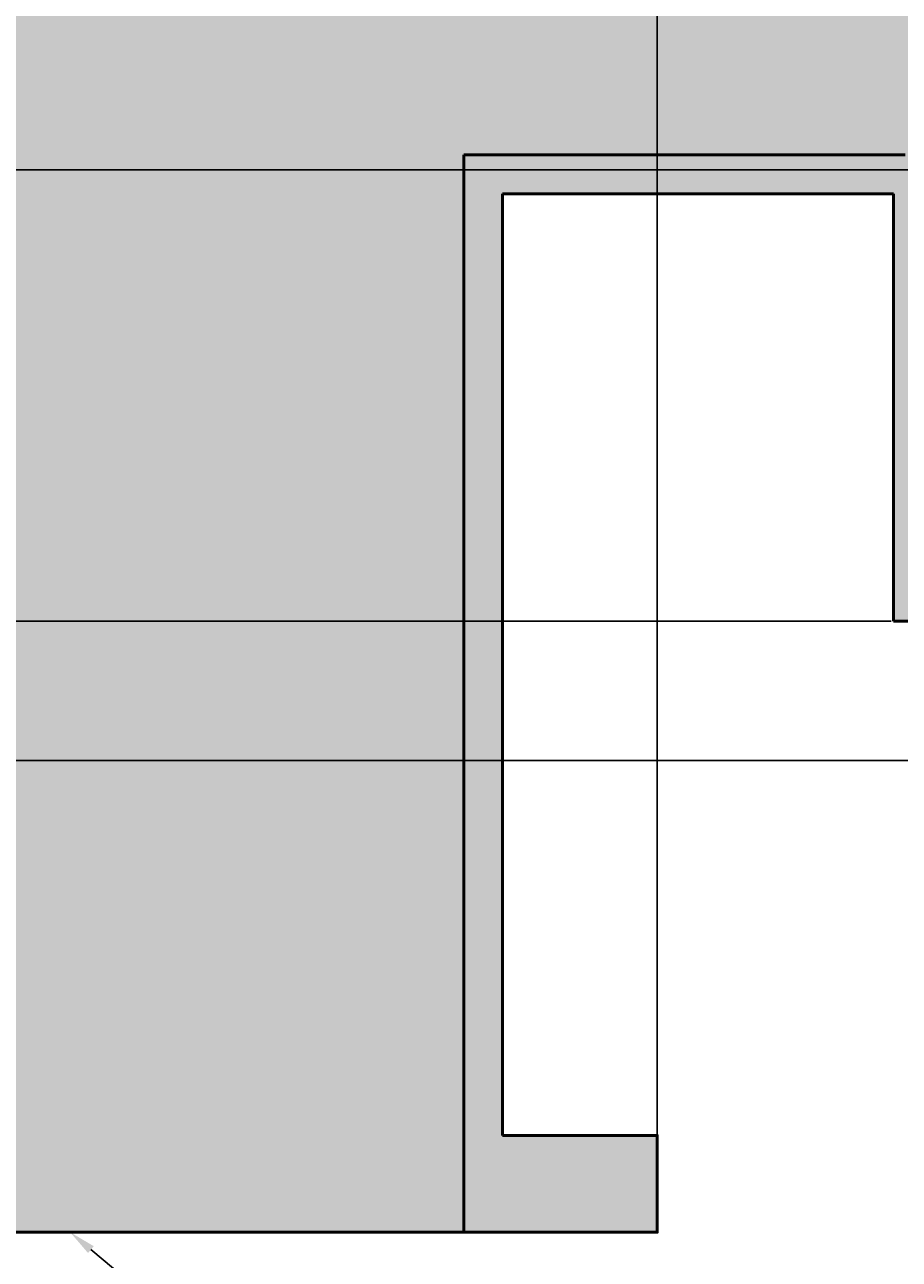
# Model space of a CAD drawing. Units: inches. Extents: x -12 to 334, y -10 to 186.
# Tile 12 of 77: x 42 to 64, y 33 to 65. Entities that reach past the tile are written whole.
import ezdxf
from ezdxf import colors
from ezdxf.entities.mleader import LeaderData, LeaderLine
from ezdxf.math import Vec2, Vec3

# ---------------------------------------------------------------- set-up
doc = ezdxf.new("R2010")
doc.units = ezdxf.units.IN
doc.header["$MEASUREMENT"] = 0
for name, color, linetype, lineweight in [('M-ANNO-TEXT', 3, 'Continuous', 25), ('M-DIMS', 2, 'Continuous', 18), ('M-EQPM', 7, 'Continuous', 50), ('M-EQPM-PATT', 8, 'Continuous', 18)]:
    doc.layers.add(name, color=color, linetype=linetype, lineweight=lineweight)
doc.styles.get("Standard").update_dxf_attribs({"font": 'arial.ttf'})
doc.dimstyles.get("Standard").update_dxf_attribs({"dimtxt": 0.18, "dimasz": 0.18, "dimexe": 0.18, "dimexo": 0.0625, "dimgap": 0.09, "dimtad": 0, "dimtih": 1, "dimtoh": 1, "dimdec": 4, "dimzin": 0, "dimdsep": 46, "dimtxsty": 'Standard', "dimcen": 0.09, "dimadec": 0, "dimazin": 0, "dimtfac": 1, "dimtdec": 4, "dimtofl": 0, "dimtmove": 0, "dimatfit": 3, "dimfxl": 1, "dimtolj": 1, "dimtzin": 0, "dimarcsym": 0})

# ---------------------------------------------------------------- blocks, each defined once
blk = doc.blocks.new('*D1')
at = {"layer": 'Defpoints', "color": 0, "transparency": 16777216}
for p in [(281.426, 91.899), (3.376, 80.692), (281.426, 14.304)]:
    blk.add_point(p, dxfattribs=at)
at = {"layer": 'M-DIMS', "color": 0, "lineweight": -2, "transparency": 16777216}
for p, q in [((281.426, 91.836), (281.426, 14.124)), ((3.376, 80.629), (3.376, 14.124)), ((3.556, 14.304), (141.935, 14.304)), ((281.246, 14.304), (142.867, 14.304))]:
    blk.add_line(p, q, dxfattribs=at)
at = {"layer": 'M-DIMS', "color": 0, "transparency": 16777216}
for points in [[(3.556, 14.334), (3.556, 14.274), (3.376, 14.304)], [(281.246, 14.334), (281.246, 14.274), (281.426, 14.304)]]:
    blk.add_solid(points, dxfattribs=at)
at = {"layer": 'M-DIMS', "color": 0, "transparency": 16777216, "insert": (142.401, 14.304), "char_height": 0.18, "attachment_point": 5}
blk.add_mtext('\\A1;278.05', dxfattribs=at)
blk = doc.blocks.new('*D14')
at = {"layer": 'Defpoints', "color": 0, "transparency": 16777216}
for p in [(63.5, 109.058), (-11.174, 49.45), (64.207, 49.45)]:
    blk.add_point(p, dxfattribs=at)
at = {"layer": 'M-DIMS', "color": 0, "lineweight": -2, "transparency": 16777216}
for p, q in [((63.438, 109.058), (-11.354, 109.058)), ((-11.174, 108.878), (-11.174, 79.436)), ((-11.174, 49.63), (-11.174, 79.072)), ((64.144, 49.45), (-11.354, 49.45))]:
    blk.add_line(p, q, dxfattribs=at)
at = {"layer": 'M-DIMS', "color": 0, "transparency": 16777216}
for points in [[(-11.204, 108.878), (-11.144, 108.878), (-11.174, 109.058)], [(-11.204, 49.63), (-11.144, 49.63), (-11.174, 49.45)]]:
    blk.add_solid(points, dxfattribs=at)
at = {"layer": 'M-DIMS', "color": 0, "transparency": 16777216, "insert": (-11.174, 79.254), "char_height": 0.18, "attachment_point": 5}
blk.add_mtext('\\A1;59.61', dxfattribs=at)
blk = doc.blocks.new('*D26')
at = {"layer": 'Defpoints', "color": 0, "transparency": 16777216}
for p in [(87.888, 169.385), (87.888, 56.321), (58.1, 33.675)]:
    blk.add_point(p, dxfattribs=at)
at = {"layer": 'M-DIMS', "color": 0, "lineweight": -2, "transparency": 16777216}
for p, q in [((58.1, 33.738), (58.1, 169.565)), ((58.28, 169.385), (72.599, 169.385)), ((87.708, 169.385), (73.389, 169.385)), ((87.888, 56.383), (87.888, 169.565))]:
    blk.add_line(p, q, dxfattribs=at)
at = {"layer": 'M-DIMS', "color": 0, "transparency": 16777216}
for points in [[(58.28, 169.415), (58.28, 169.355), (58.1, 169.385)], [(87.708, 169.415), (87.708, 169.355), (87.888, 169.385)]]:
    blk.add_solid(points, dxfattribs=at)
at = {"layer": 'M-DIMS', "color": 0, "transparency": 16777216, "insert": (72.994, 169.385), "char_height": 0.18, "attachment_point": 5}
blk.add_mtext('\\A1;29.79', dxfattribs=at)
blk = doc.blocks.new('*D29')
at = {"layer": 'Defpoints', "color": 0, "transparency": 16777216}
for p in [(-11.174, 45.854), (221.576, 45.854), (216.576, 30.854)]:
    blk.add_point(p, dxfattribs=at)
at = {"layer": 'M-DIMS', "color": 0, "lineweight": -2, "transparency": 16777216}
for p, q in [((221.514, 45.854), (-11.354, 45.854)), ((-11.174, 45.674), (-11.174, 38.536)), ((-11.174, 31.034), (-11.174, 38.172)), ((216.514, 30.854), (-11.354, 30.854))]:
    blk.add_line(p, q, dxfattribs=at)
at = {"layer": 'M-DIMS', "color": 0, "transparency": 16777216}
for points in [[(-11.204, 45.674), (-11.144, 45.674), (-11.174, 45.854)], [(-11.204, 31.034), (-11.144, 31.034), (-11.174, 30.854)]]:
    blk.add_solid(points, dxfattribs=at)
at = {"layer": 'M-DIMS', "color": 0, "transparency": 16777216, "insert": (-11.174, 38.354), "char_height": 0.18, "attachment_point": 5}
blk.add_mtext('\\A1;15', dxfattribs=at)
blk = doc.blocks.new('*D35')
at = {"layer": 'Defpoints', "color": 0, "transparency": 16777216}
for p in [(216.428, 98.108), (-11.174, 61.105), (216.428, 61.105)]:
    blk.add_point(p, dxfattribs=at)
at = {"layer": 'M-DIMS', "color": 0, "lineweight": -2, "transparency": 16777216}
for p, q in [((216.365, 98.108), (-11.354, 98.108)), ((-11.174, 97.928), (-11.174, 79.788)), ((-11.174, 61.285), (-11.174, 79.424)), ((216.365, 61.105), (-11.354, 61.105))]:
    blk.add_line(p, q, dxfattribs=at)
at = {"layer": 'M-DIMS', "color": 0, "transparency": 16777216}
for points in [[(-11.204, 97.928), (-11.144, 97.928), (-11.174, 98.108)], [(-11.204, 61.285), (-11.144, 61.285), (-11.174, 61.105)]]:
    blk.add_solid(points, dxfattribs=at)
at = {"layer": 'M-DIMS', "color": 0, "transparency": 16777216, "insert": (-11.174, 79.606), "char_height": 0.18, "attachment_point": 5}
blk.add_mtext('\\A1;37', dxfattribs=at)
blk = doc.blocks.new('*D39')
at = {"layer": 'Defpoints', "color": 0, "transparency": 16777216}
for p in [(279.726, 80.692), (-11.174, 45.854), (269.381, 45.854)]:
    blk.add_point(p, dxfattribs=at)
at = {"layer": 'M-DIMS', "color": 0, "lineweight": -2, "transparency": 16777216}
for p, q in [((279.664, 80.692), (-11.354, 80.692)), ((-11.174, 80.512), (-11.174, 63.455)), ((-11.174, 46.034), (-11.174, 63.091)), ((269.318, 45.854), (-11.354, 45.854))]:
    blk.add_line(p, q, dxfattribs=at)
at = {"layer": 'M-DIMS', "color": 0, "transparency": 16777216}
for points in [[(-11.204, 80.512), (-11.144, 80.512), (-11.174, 80.692)], [(-11.204, 46.034), (-11.144, 46.034), (-11.174, 45.854)]]:
    blk.add_solid(points, dxfattribs=at)
at = {"layer": 'M-DIMS', "color": 0, "transparency": 16777216, "insert": (-11.174, 63.273), "char_height": 0.18, "attachment_point": 5}
blk.add_mtext('\\A1;34.84', dxfattribs=at)

msp = doc.modelspace()

# ---------------------------------------------------------------- hatches: boundary and pattern name
at = {"layer": 'M-EQPM-PATT'}
h = msp.add_hatch(color=256, dxfattribs=at)
h.set_gradient(color1=(99, 100, 102), color2=(99, 100, 102), tint=1)
h.paths.add_polyline_path([(4.3766, 80.754, -0.4132606), (23.5807, 99.8958), (37.1002, 99.8958), (37.1002, 127.7078), (32.1002, 127.7078), (32.1002, 125.2078), (36.1002, 125.2078), (36.1002, 100.8958), (23.5807, 100.8958, 1), (23.5807, 60.4872), (36.1002, 60.4872), (36.1002, 36.1752), (32.1002, 36.1752), (32.1002, 33.6752), (37.1002, 33.6752), (37.1002, 61.4872), (23.5807, 61.4872, -0.384914), (4.4744, 78.754), (72.9244, 78.754), (72.9244, 69.6117), (75.9244, 69.6117), (75.9244, 89.8963), (72.9244, 89.8963), (72.9244, 80.754)])
h.paths.add_polyline_path([(54.1002, 125.2078), (58.1002, 125.2078), (58.1002, 127.7078), (53.1002, 127.7078), (53.1002, 99.8958), (64.5, 99.8958), (64.5, 109.0583), (63.5, 109.0583), (63.5, 100.8958), (54.1002, 100.8958)], flags=17)
h.paths.add_polyline_path([(53.1002, 33.6752), (58.1002, 33.6752), (58.1002, 36.1752), (54.1002, 36.1752), (54.1002, 60.4872), (64.2068, 60.4872), (64.2068, 49.4497), (87.8879, 49.4497), (87.8879, 55.3205), (104.8919, 55.3205), (104.8919, 30.8541), (99.8919, 30.8541), (99.8919, 28.8541), (105.8919, 28.8541), (105.8919, 56.3205), (87.8879, 56.3205), (87.8879, 63.6117), (86.8879, 63.6117), (86.8879, 50.4497), (65.0061, 50.4497), (65.0061, 63.6117), (64.5, 63.6117), (64.5, 61.4872), (53.1002, 61.4872)])
h.paths.add_polyline_path([(121.8919, 28.8541), (121.8919, 30.8541), (116.8919, 30.8541), (116.8919, 45.8541), (209.6965, 45.8541), (209.9204, 46.8541), (115.8919, 46.8541), (115.8919, 28.8541)])
h.paths.add_polyline_path([(221.5761, 32.8541), (216.5761, 32.8541), (216.5761, 30.8541), (222.5761, 30.8541), (222.5761, 46.8541), (209.9204, 46.8541), (209.6965, 45.8541), (221.5761, 45.8541)])
h.paths.add_polyline_path([(233.5761, 45.8541), (249.8485, 45.8541), (249.3759, 46.8541), (232.5761, 46.8541), (232.5761, 30.8541), (238.5761, 30.8541), (238.5761, 32.8541), (233.5761, 32.8541)])
h = msp.add_hatch(color=256, dxfattribs=at)
h.set_gradient(color1=(205, 32, 39), color2=(205, 32, 39), tint=1)
h.paths.add_polyline_path([(64.5, 80.754), (64.5, 89.8963), (226.6083, 89.8963, -1), (226.6083, 69.6117), (64.5, 69.6117), (64.5, 78.754), (4.4744, 78.754, 0.384914), (23.5807, 61.4872), (37.1002, 61.4872), (37.1002, 33.6752), (53.1002, 33.6752), (53.1002, 61.4872), (64.5, 61.4872), (64.5, 63.6117), (226.6083, 63.6117, 1), (226.6083, 95.8963), (64.5, 95.8963), (64.5, 99.8958), (53.1002, 99.8958), (53.1002, 127.7078), (37.1002, 127.7078), (37.1002, 99.8958), (23.5807, 99.8958, 0.4132606), (4.3766, 80.754)])
h.paths.add_polyline_path([(64.5, 91.8963), (64.5, 93.8963), (226.6083, 93.8963, -1), (226.6083, 65.6117), (64.5, 65.6117), (64.5, 67.6117), (226.6083, 67.6117, 1), (226.6083, 91.8963)], flags=16)

# ---------------------------------------------------------------- linework, layer by layer
at = {"layer": 'M-EQPM'}
for p, q in [((53.1002, 61.4872), (53.1002, 33.6752)), ((54.1002, 60.4872), (54.1002, 36.1752)), ((64.2068, 49.4497), (64.2068, 60.4872)), ((87.8879, 49.4497), (64.2068, 49.4497))]:
    msp.add_line(p, q, dxfattribs=at)
for points in [[(64.5, 61.4872), (53.1002, 61.4872)], [(64.2068, 60.4872), (54.1002, 60.4872)], [(36.1002, 36.1752), (32.1002, 36.1752), (32.1002, 33.6752), (58.1002, 33.6752), (58.1002, 36.1752), (54.1002, 36.1752)]]:
    msp.add_lwpolyline(points, dxfattribs=at)

# ---------------------------------------------------------------- dimensions: what is measured, and where the dimension line sits
at = {"layer": 'M-DIMS'}
for base, p1, p2, picture, middle in [((87.8879, 169.3845), (58.1002, 33.6752), (87.8879, 56.3205), '*D26', (72.9941, 169.3845)), ((281.4256, 14.3041), (3.3765, 80.6915), (281.4256, 91.8988), '*D1', (142.401, 14.3041))]:
    dim = msp.add_linear_dim(base=base, p1=p1, p2=p2, dimstyle='Standard', override={"dimdec": 2, "dimlfac": 1, "dimrnd": 0, "dimzin": 0, "dimdsep": 46, "dimlunit": 2}, dxfattribs=at)
    dim.commit()
    dim.dimension.update_dxf_attribs({"geometry": picture, "text_midpoint": middle})
for base, p1, p2, override, picture, middle in [((-11.1736, 49.4497), (63.5, 109.0583), (64.2068, 49.4497), {"dimdec": 2, "dimlfac": 1, "dimrnd": 0, "dimzin": 0, "dimdsep": 46, "dimlunit": 2}, '*D14', (-11.1735, 79.254)), ((-11.1736, 61.1045), (216.4278, 98.1081), (216.4278, 61.1045), {"dimdec": 0, "dimlfac": 1, "dimrnd": 0, "dimzin": 0, "dimdsep": 46, "dimlunit": 2}, '*D35', (-11.1735, 79.6063)), ((-11.1736, 45.8541), (279.7263, 80.6915), (269.3808, 45.8541), {"dimdec": 2, "dimlfac": 1, "dimrnd": 0, "dimzin": 0, "dimdsep": 46, "dimlunit": 2}, '*D39', (-11.1735, 63.2728)), ((-11.1736, 45.8541), (216.5761, 30.8541), (221.5761, 45.8541), {"dimdec": 0, "dimlfac": 1, "dimrnd": 0, "dimzin": 0, "dimdsep": 46, "dimlunit": 2}, '*D29', (-11.1735, 38.3541))]:
    dim = msp.add_linear_dim(base=base, p1=p1, p2=p2, angle=90, dimstyle='Standard', override=override, dxfattribs=at)
    dim.commit()
    dim.dimension.update_dxf_attribs({"geometry": picture, "text_midpoint": middle})

# ---------------------------------------------------------------- leaders
at = {"layer": 'M-ANNO-TEXT'}
ml = msp.add_multileader_mtext('Standard', dxfattribs=at)
ml.set_content('^ICondensate outlet', color=256)
ml.set_leader_properties()
ml.build(insert=Vec2(0, 0))
ml.multileader.update_dxf_attribs({"dogleg_length": 0.36, "arrow_head_size": 0.7})
ctx = ml.context
ctx.base_point, ctx.arrow_head_size, ctx.landing_gap_size, ctx.plane_origin = Vec3(83.8784, 10.3512), 0.7, 0.09, Vec3(49.4251, 25.7584)
notes = []
notes.append((ctx, [(0, (1, 1, 0), (70.8242, 10.3512), (1, 0), 13.0542, [(0, [(42.9275, 33.6752)], 0, [])])]))
ctx.mtext.insert, ctx.mtext.flow_direction = Vec3(83.9684, 12.3853), 5
for ctx, leaders in notes:
    for number, flags, end, landing, length, lines in leaders:
        leader = LeaderData()
        leader.index, (leader.has_last_leader_line, leader.has_dogleg_vector, leader.attachment_direction) = number, flags
        leader.last_leader_point, leader.dogleg_vector, leader.dogleg_length = Vec3(end), Vec3(landing), length
        for number, points, colour, breaks in lines:
            line = LeaderLine()
            line.index, line.vertices, line.color, line.breaks = number, Vec3.list(points), colors.encode_raw_color(colour), breaks
            leader.lines.append(line)
        ctx.leaders.append(leader)

doc.saveas('drawing.dxf')
